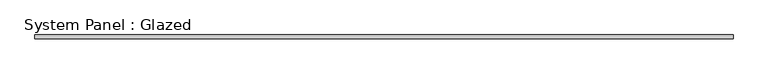
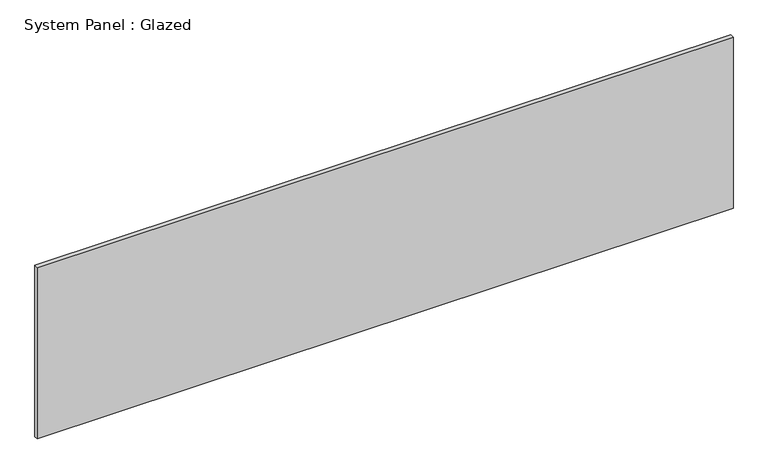
"""IFC4 building model written with IfcOpenShell, lengths in millimetres: plate geometry, System Panel : Glazed."""

from ifc_helpers import new_model, si_unit, origin, origin_with_axes, place, context, project, spatial, polyline, outline, extrude, source, transform, mapped, element, save


def system_panel_glazed_62bdce80(model_context):
    return source(origin(), model_context, "Body", "SweptSolid", [
        extrude(outline(polyline([(2344.1734365, 19.05), (-2344.1734365, 19.05), (-2344.1734365, 44.45), (2344.1734365, 44.45), (2344.1734365, 19.05)])), origin_with_axes(), (0.0, 0.0, 1.0), 1219.2),
    ])


if __name__ == "__main__":
    model = new_model("IFC4")
    model_context = context("Model", 3, world=origin())
    ifc_project = project(units=[si_unit("LENGTHUNIT", "METRE", prefix="MILLI")], contexts=[model_context])
    site = spatial("IfcSite", under=ifc_project)
    building = spatial("IfcBuilding", under=site)
    placement = place(None, origin())
    system_panel_glazed_shape = system_panel_glazed_62bdce80(model_context)
    element("IfcPlate", 1, ObjectType="System Panel : Glazed", at=placement, inside=building, context=model_context, shape_type="MappedRepresentation", body=[
        mapped(system_panel_glazed_shape, transform((0.0, 0.0, 0.0), x_axis=(1.0, 0.0, 0.0), y_axis=(0.0, 1.0, 0.0), z_axis=(0.0, 0.0, 1.0))),
    ])
    save(model, "model.ifc")

# Revit data of these elements
# Type "System Panel : Glazed"
#   Construction Type Id = "GSP4R"
#   Analytic Construction = "1/8 in Pilkington single glazing"
#   Visual Light Transmittance = 0.9
#   Solar Heat Gain Coefficient = 0.86
#   Heat Transfer Coefficient (U) = 1.18115 BTU/(h·ft²·°F)
# Element 1 (IfcPlate, "System Panel : Glazed")
#   Materials on its faces: "Glass"
# Materials
#   "Glass": class "Glass", colour RGB 0 128 192, transparency 0.75, Description = "Soda Lime Glass", Cost = 0
